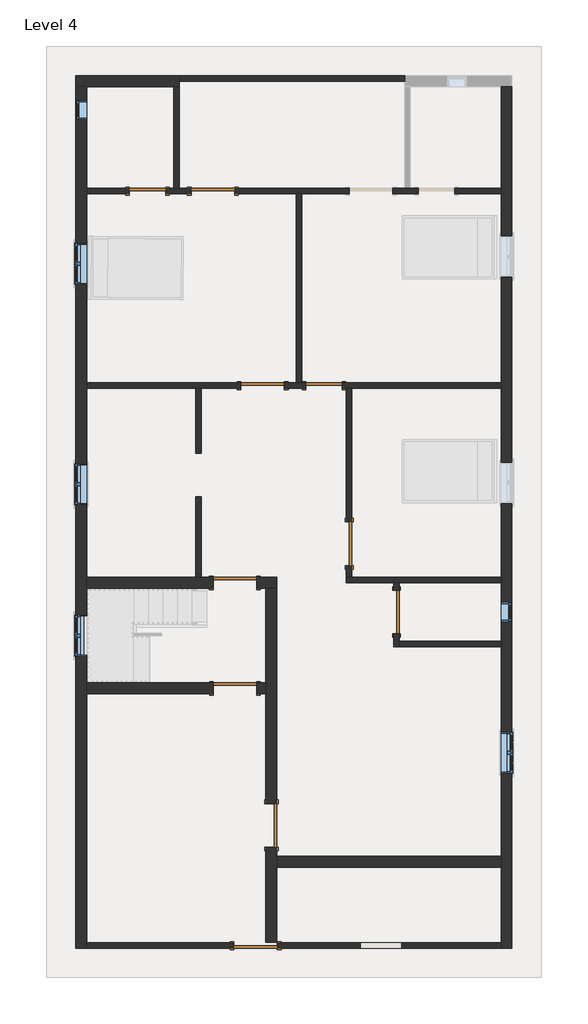
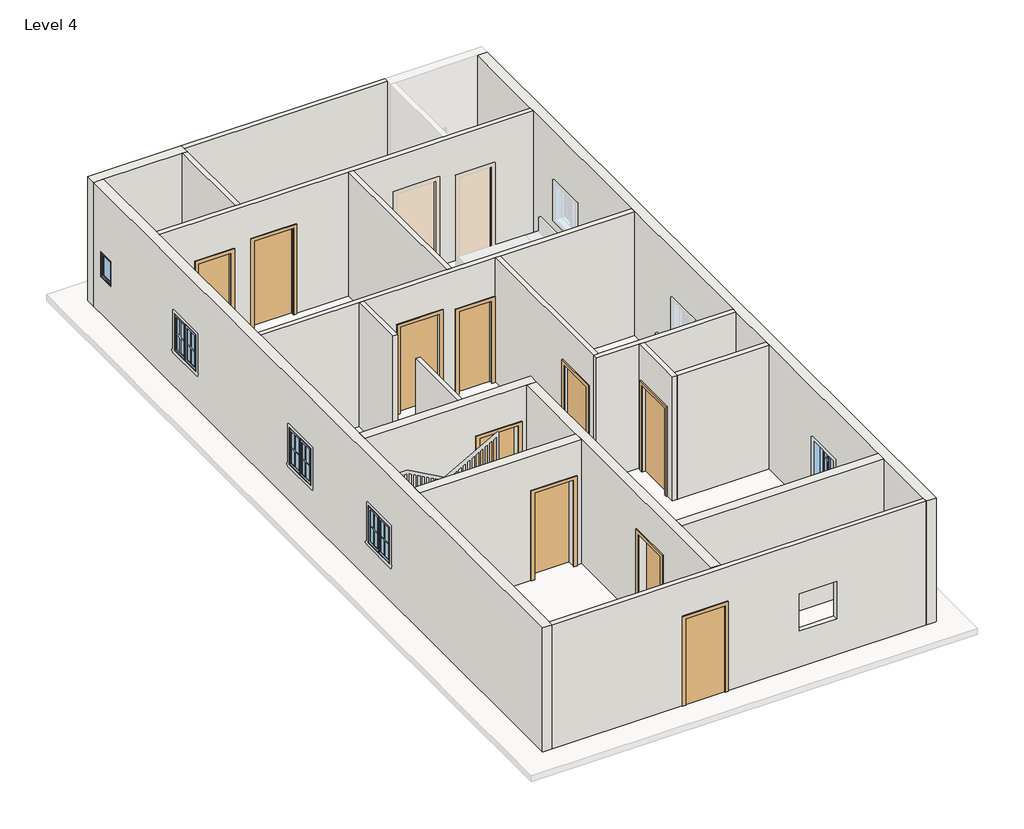
# One storey, part 1 of 3: 19 walls, 10 doors, 6 windows.
"""IFC4 building model written with IfcOpenShell, lengths in millimetres."""

from ifc_helpers import new_model, si_unit, frame, origin, place, context, project, spatial, polyline, outline, extrude, faceted_brep, transform, mapped, element, save
from components import door_d8f5dbb5, door_f2b275c1, door_e5f9f3c4, door_0ca8825f, door_305aa2a5, window_aa618e30, window_339605e1

model = new_model("IFC4")

# Units and contexts
model_context = context("Model", 3, world=origin())
ifc_project = project(units=[si_unit("LENGTHUNIT", "METRE", prefix="MILLI")], contexts=[model_context])

# Site, building, storey
site = spatial("IfcSite", under=ifc_project)
building = spatial("IfcBuilding", under=site)
storey = spatial("IfcBuildingStorey", under=building, Name="Level 4", Elevation=6400.8)

# Doors
placement = place(None, origin())
door_shape = door_d8f5dbb5(model_context)
element("IfcDoor", 1, ObjectType="Single-Flush : 30\" x 80\"", at=placement, inside=storey, context=model_context, shape_type="MappedRepresentation", body=[
    mapped(door_shape, transform((-4322.2915084, 8007.7072267, 6400.8), x_axis=(1.0, 0.0, 0.0), y_axis=(0.0, 1.0, 0.0), z_axis=(0.0, 0.0, 1.0))),
])
door_2_shape = door_f2b275c1(model_context)
element("IfcDoor", 2, ObjectType="Single-Flush : 30\" x 80\"", at=placement, inside=storey, context=model_context, shape_type="MappedRepresentation", body=[
    mapped(door_2_shape, transform((-621.124692, 3931.0072267, 6400.8), x_axis=(-1.0, 0.0, 0.0), y_axis=(0.0, -1.0, 0.0), z_axis=(0.0, 0.0, 1.0))),
])
door_3_shape = door_e5f9f3c4(model_context)
element("IfcDoor", 3, ObjectType="Single-Flush : 36\" x 84\"", at=placement, inside=storey, context=model_context, shape_type="MappedRepresentation", body=[
    mapped(door_3_shape, transform((-1909.2915084, 3931.0072267, 6400.8), x_axis=(1.0, 0.0, 0.0), y_axis=(0.0, 1.0, 0.0), z_axis=(0.0, 0.0, 1.0))),
])
element("IfcDoor", 4, ObjectType="Single-Flush : 36\" x 84\"", at=placement, inside=storey, context=model_context, shape_type="MappedRepresentation", body=[
    mapped(door_3_shape, transform((-94.9578757, 616.3072267, 6400.8), x_axis=(0.0, -1.0, 0.0), y_axis=(1.0, 0.0, 0.0), z_axis=(0.0, 0.0, 1.0))),
])
element("IfcDoor", 5, ObjectType="Single-Flush : 36\" x 84\"", at=placement, inside=storey, context=model_context, shape_type="MappedRepresentation", body=[
    mapped(door_3_shape, transform((-2055.3415084, -7803.7927733, 6400.8), x_axis=(-1.0, 0.0, 0.0), y_axis=(0.0, -1.0, 0.0), z_axis=(0.0, 0.0, 1.0))),
])
door_4_shape = door_0ca8825f(model_context)
element("IfcDoor", 6, ObjectType="Single-Flush : 36\" x 84\"", at=placement, inside=storey, context=model_context, shape_type="MappedRepresentation", body=[
    mapped(door_4_shape, transform((-2490.3165084, -202.8427733, 6400.8), x_axis=(1.0, 0.0, 0.0), y_axis=(0.0, 1.0, 0.0), z_axis=(0.0, 0.0, 1.0))),
])
element("IfcDoor", 7, ObjectType="Single-Flush : 36\" x 84\"", at=placement, inside=storey, context=model_context, shape_type="MappedRepresentation", body=[
    mapped(door_4_shape, transform((-2487.1415084, -2412.6427733, 6400.8), x_axis=(1.0, 0.0, 0.0), y_axis=(0.0, 1.0, 0.0), z_axis=(0.0, 0.0, 1.0))),
])
element("IfcDoor", 8, ObjectType="Single-Flush : 36\" x 84\"", at=placement, inside=storey, context=model_context, shape_type="MappedRepresentation", body=[
    mapped(door_4_shape, transform((-1725.1415084, -5282.8427733, 6400.8), x_axis=(0.0, -1.0, 0.0), y_axis=(1.0, 0.0, 0.0), z_axis=(0.0, 0.0, 1.0))),
])
door_5_shape = door_305aa2a5(model_context)
element("IfcDoor", 9, ObjectType="Single-Flush : 36\" x 84\"", at=placement, inside=storey, context=model_context, shape_type="MappedRepresentation", body=[
    mapped(door_5_shape, transform((897.4084916, -812.4427733, 6400.8), x_axis=(0.0, 1.0, 0.0), y_axis=(-1.0, 0.0, 0.0), z_axis=(0.0, 0.0, 1.0))),
])
element("IfcDoor", 10, ObjectType="Single-Flush : 36\" x 84\"", at=placement, inside=storey, context=model_context, shape_type="MappedRepresentation", body=[
    mapped(door_5_shape, transform((-2950.6915084, 8007.7072267, 6400.8), x_axis=(-1.0, 0.0, 0.0), y_axis=(0.0, -1.0, 0.0), z_axis=(0.0, 0.0, 1.0))),
])

# Walls
element("IfcWall", 11, ObjectType="WALL4.5\"", at=placement, inside=storey, context=model_context, shape_type="Brep", body=[
    faceted_brep([(821.2084916, 7950.5572267, 8534.4), (821.2084916, 7950.5572267, 6400.8), (1354.6084916, 7950.5572267, 6400.8), (1354.6084916, 7950.5572267, 8432.8), (2116.6084916, 7950.5572267, 8432.8), (2116.6084916, 7950.5572267, 6400.8), (3088.1584916, 7950.5572267, 6400.8), (3088.1584916, 7950.5572267, 9448.8), (-1090.1415084, 7950.5572267, 9448.8), (-1204.4415084, 7950.5572267, 9448.8), (-5598.6415084, 7950.5572267, 9448.8), (-5598.6415084, 7950.5572267, 6400.8), (-4703.2915084, 7950.5572267, 6400.8), (-4703.2915084, 7950.5572267, 8432.8), (-3941.2915084, 7950.5572267, 8432.8), (-3941.2915084, 7950.5572267, 6400.8), (-3407.8915084, 7950.5572267, 6400.8), (-3407.8915084, 7950.5572267, 8534.4), (-2493.4915084, 7950.5572267, 8534.4), (-2493.4915084, 7950.5572267, 6400.8), (-1204.4415084, 7950.5572267, 6400.8), (-1090.1415084, 7950.5572267, 6400.8), (-93.1915084, 7950.5572267, 6400.8), (-93.1915084, 7950.5572267, 8534.4), (1354.6084916, 8064.8572267, 6400.8), (1183.1584916, 8064.8572267, 6400.8), (1068.8584916, 8064.8572267, 6400.8), (821.2084916, 8064.8572267, 6400.8), (821.2084916, 8064.8572267, 8534.4), (-93.1915084, 8064.8572267, 8534.4), (-93.1915084, 8064.8572267, 6400.8), (-2493.4915084, 8064.8572267, 6400.8), (-2493.4915084, 8064.8572267, 8534.4), (-3407.8915084, 8064.8572267, 8534.4), (-3407.8915084, 8064.8572267, 6400.8), (-3655.5415084, 8064.8572267, 6400.8), (-3769.8415084, 8064.8572267, 6400.8), (-3941.2915084, 8064.8572267, 6400.8), (-3941.2915084, 8064.8572267, 8432.8), (-4703.2915084, 8064.8572267, 8432.8), (-4703.2915084, 8064.8572267, 6400.8), (-5598.6415084, 8064.8572267, 6400.8), (-5598.6415084, 8064.8572267, 9448.8), (-3769.8415084, 8064.8572267, 9448.8), (-3655.5415084, 8064.8572267, 9448.8), (1068.8584916, 8064.8572267, 9448.8), (1183.1584916, 8064.8572267, 9448.8), (3088.1584916, 8064.8572267, 9448.8), (3088.1584916, 8064.8572267, 6400.8), (2116.6084916, 8064.8572267, 6400.8), (2116.6084916, 8064.8572267, 8432.8), (1354.6084916, 8064.8572267, 8432.8)], [[[0, 1, 2, 3, 4, 5, 6, 7, 8, 9, 10, 11, 12, 13, 14, 15, 16, 17, 18, 19, 20, 21, 22, 23]], [[24, 25, 26, 27, 28, 29, 30, 31, 32, 33, 34, 35, 36, 37, 38, 39, 40, 41, 42, 43, 44, 45, 46, 47, 48, 49, 50, 51]], [[12, 11, 41, 40]], [[49, 48, 6, 5]], [[37, 36, 35, 34, 16, 15]], [[2, 1, 27, 26, 25, 24]], [[22, 21, 20, 19, 31, 30]], [[11, 10, 42, 41]], [[7, 6, 48, 47]], [[38, 37, 15, 14]], [[39, 38, 14, 13]], [[40, 39, 13, 12]], [[3, 2, 24, 51]], [[4, 3, 51, 50]], [[5, 4, 50, 49]], [[17, 16, 34, 33]], [[18, 17, 33, 32]], [[19, 18, 32, 31]], [[28, 27, 1, 0]], [[29, 28, 0, 23]], [[30, 29, 23, 22]], [[10, 9, 8, 7, 47, 46, 45, 44, 43, 42]]]),
])
element("IfcWall", 12, ObjectType="WALL4.5\"", at=placement, inside=storey, context=model_context, shape_type="SweptSolid", body=[
    extrude(outline(polyline([(-3769.8415084, 8064.8572267), (-3769.8415084, 10198.4572267), (-3655.5415084, 10198.4572267), (-3655.5415084, 8064.8572267), (-3769.8415084, 8064.8572267)])), frame((0.0, 0.0, 6400.8), z_axis=(0.0, 0.0, 1.0), x_axis=(1.0, 0.0, 0.0)), (0.0, 0.0, 1.0), 3048.0),
])
element("IfcWall", 13, ObjectType="WALL4.5\"", at=placement, inside=storey, context=model_context, shape_type="SweptSolid", body=[
    extrude(outline(polyline([(-1204.4415084, 3988.1572267), (-1204.4415084, 7950.5572267), (-1090.1415084, 7950.5572267), (-1090.1415084, 3988.1572267), (-1204.4415084, 3988.1572267)])), frame((0.0, 0.0, 6400.8), z_axis=(0.0, 0.0, 1.0), x_axis=(1.0, 0.0, 0.0)), (0.0, 0.0, 1.0), 3048.0),
])
element("IfcWall", 14, ObjectType="WALL4.5\"", at=placement, inside=storey, context=model_context, shape_type="Brep", body=[
    faceted_brep([(-1452.0915084, 3873.8572267, 6400.8), (-1002.124692, 3873.8572267, 6400.8), (-1002.124692, 3873.8572267, 8432.8), (-240.124692, 3873.8572267, 8432.8), (-240.124692, 3873.8572267, 6400.8), (-152.1078757, 3873.8572267, 6400.8), (-37.8078757, 3873.8572267, 6400.8), (3088.1584916, 3873.8572267, 6400.8), (3088.1584916, 3873.8572267, 9448.8), (-37.8078757, 3873.8572267, 9448.8), (-152.1078757, 3873.8572267, 9448.8), (-3198.3415084, 3873.8572267, 9448.8), (-3312.6415084, 3873.8572267, 9448.8), (-5598.6415084, 3873.8572267, 9448.8), (-5598.6415084, 3873.8572267, 6400.8), (-3312.6415084, 3873.8572267, 6400.8), (-3198.3415084, 3873.8572267, 6400.8), (-2366.4915084, 3873.8572267, 6400.8), (-2366.4915084, 3873.8572267, 8534.4), (-1452.0915084, 3873.8572267, 8534.4), (-1002.124692, 3988.1572267, 8432.8), (-1002.124692, 3988.1572267, 6400.8), (-1090.1415084, 3988.1572267, 6400.8), (-1204.4415084, 3988.1572267, 6400.8), (-1452.0915084, 3988.1572267, 6400.8), (-1452.0915084, 3988.1572267, 8534.4), (-2366.4915084, 3988.1572267, 8534.4), (-2366.4915084, 3988.1572267, 6400.8), (-5598.6415084, 3988.1572267, 6400.8), (-5598.6415084, 3988.1572267, 9448.8), (-1204.4415084, 3988.1572267, 9448.8), (-1090.1415084, 3988.1572267, 9448.8), (3088.1584916, 3988.1572267, 9448.8), (3088.1584916, 3988.1572267, 6400.8), (-240.124692, 3988.1572267, 6400.8), (-240.124692, 3988.1572267, 8432.8)], [[[0, 1, 2, 3, 4, 5, 6, 7, 8, 9, 10, 11, 12, 13, 14, 15, 16, 17, 18, 19]], [[20, 21, 22, 23, 24, 25, 26, 27, 28, 29, 30, 31, 32, 33, 34, 35]], [[17, 16, 15, 14, 28, 27]], [[34, 33, 7, 6, 5, 4]], [[24, 23, 22, 21, 1, 0]], [[14, 13, 29, 28]], [[8, 7, 33, 32]], [[25, 24, 0, 19]], [[26, 25, 19, 18]], [[27, 26, 18, 17]], [[2, 1, 21, 20]], [[3, 2, 20, 35]], [[4, 3, 35, 34]], [[13, 12, 11, 10, 9, 8, 32, 31, 30, 29]]]),
])
element("IfcWall", 15, ObjectType="WALL4.5\"", at=placement, inside=storey, context=model_context, shape_type="SweptSolid", body=[
    extrude(outline(polyline([(-3312.6415084, 2514.5843832), (-3312.6415084, 3873.8572267), (-3198.3415084, 3873.8572267), (-3198.3415084, 2514.5843832), (-3312.6415084, 2514.5843832)])), frame((0.0, 0.0, 6400.8), z_axis=(0.0, 0.0, 1.0), x_axis=(1.0, 0.0, 0.0)), (0.0, 0.0, 1.0), 3048.0),
])
element("IfcWall", 16, ObjectType="WALL4.5\"", at=placement, inside=storey, context=model_context, shape_type="SweptSolid", body=[
    extrude(outline(polyline([(-3312.6415084, -88.5427733), (-3312.6415084, 1600.2092553), (-3198.3415084, 1600.2092553), (-3198.3415084, -88.5427733), (-3312.6415084, -88.5427733)])), frame((0.0, 0.0, 6400.8), z_axis=(0.0, 0.0, 1.0), x_axis=(1.0, 0.0, 0.0)), (0.0, 0.0, 1.0), 3048.0),
])
element("IfcWall", 17, ObjectType="WALL4.5\"", at=placement, inside=storey, context=model_context, shape_type="SweptSolid", body=[
    extrude(outline(polyline([(159.1072267, 8534.4), (159.1072267, 6400.8), (-88.5427733, 6400.8), (-88.5427733, 9448.8), (3873.8572267, 9448.8), (3873.8572267, 6400.8), (1073.5072267, 6400.8), (1073.5072267, 8534.4), (159.1072267, 8534.4)])), frame((-152.1078757, 0.0, 0.0), z_axis=(1.0, 0.0, 0.0), x_axis=(0.0, 1.0, 0.0)), (0.0, 0.0, 1.0), 114.3),
])
element("IfcWall", 18, ObjectType="WALL4.5\"", at=placement, inside=storey, context=model_context, shape_type="Brep", body=[
    faceted_brep([(-152.1078757, -202.8427733, 6400.8), (840.2584916, -202.8427733, 6400.8), (954.5584916, -202.8427733, 6400.8), (3088.1584916, -202.8427733, 6400.8), (3088.1584916, -202.8427733, 9448.8), (954.5584916, -202.8427733, 9448.8), (840.2584916, -202.8427733, 9448.8), (-152.1078757, -202.8427733, 9448.8), (-152.1078757, -88.5427733, 6400.8), (-152.1078757, -88.5427733, 9448.8), (-37.8078757, -88.5427733, 9448.8), (3088.1584916, -88.5427733, 9448.8), (3088.1584916, -88.5427733, 6400.8), (-37.8078757, -88.5427733, 6400.8)], [[[0, 1, 2, 3, 4, 5, 6, 7]], [[8, 9, 10, 11, 12, 13]], [[3, 2, 1, 0, 8, 13, 12]], [[4, 3, 12, 11]], [[0, 7, 9, 8]], [[7, 6, 5, 4, 11, 10, 9]]]),
])
element("IfcWall", 19, ObjectType="WALL4.5\"", at=placement, inside=storey, context=model_context, shape_type="Brep", body=[
    faceted_brep([(840.2584916, -202.8427733, 6400.8), (840.2584916, -355.2427733, 6400.8), (840.2584916, -355.2427733, 8534.4), (840.2584916, -1269.6427733, 8534.4), (840.2584916, -1269.6427733, 6400.8), (840.2584916, -1536.3427733, 6400.8), (840.2584916, -1536.3427733, 9448.8), (840.2584916, -202.8427733, 9448.8), (954.5584916, -355.2427733, 8534.4), (954.5584916, -355.2427733, 6400.8), (954.5584916, -202.8427733, 6400.8), (954.5584916, -202.8427733, 9448.8), (954.5584916, -1422.0427733, 9448.8), (954.5584916, -1536.3427733, 9448.8), (954.5584916, -1536.3427733, 6400.8), (954.5584916, -1422.0427733, 6400.8), (954.5584916, -1269.6427733, 6400.8), (954.5584916, -1269.6427733, 8534.4)], [[[0, 1, 2, 3, 4, 5, 6, 7]], [[8, 9, 10, 11, 12, 13, 14, 15, 16, 17]], [[10, 9, 1, 0]], [[16, 15, 14, 5, 4]], [[0, 7, 11, 10]], [[6, 5, 14, 13]], [[2, 1, 9, 8]], [[3, 2, 8, 17]], [[4, 3, 17, 16]], [[7, 6, 13, 12, 11]]]),
])
element("IfcWall", 20, ObjectType="WALL4.5\"", at=placement, inside=storey, context=model_context, shape_type="SweptSolid", body=[
    extrude(outline(polyline([(3088.1584916, -1536.3427733), (954.5584916, -1536.3427733), (954.5584916, -1422.0427733), (3088.1584916, -1422.0427733), (3088.1584916, -1536.3427733)])), frame((0.0, 0.0, 6400.8), z_axis=(0.0, 0.0, 1.0), x_axis=(1.0, 0.0, 0.0)), (0.0, 0.0, 1.0), 3048.0),
])
element("IfcWall", 21, ObjectType="WALL4.5\"", at=placement, inside=storey, context=model_context, shape_type="SweptSolid", body=[
    extrude(outline(polyline([(6400.8, -5598.6415084), (6400.8, -2512.5415084), (8534.4, -2512.5415084), (8534.4, -1598.1415084), (6400.8, -1598.1415084), (6400.8, 3088.1584916), (9448.8, 3088.1584916), (9448.8, -5598.6415084), (6400.8, -5598.6415084)]), holes=[polyline([(8199.7190366, 141.7584916), (8199.7190366, 1005.3584916), (7285.3190366, 1005.3584916), (7285.3190366, 141.7584916), (8199.7190366, 141.7584916)])]), frame((0.0, -7860.9427733, 0.0), z_axis=(0.0, 1.0, 0.0), x_axis=(0.0, 0.0, 1.0)), (0.0, 0.0, 1.0), 114.3),
])
element("IfcWall", 22, ObjectType="WALL4.5\"", at=placement, inside=storey, context=model_context, shape_type="SweptSolid", body=[
    extrude(outline(polyline([(1068.8584916, 10312.7572267), (-3655.5415084, 10312.7572267), (-3655.5415084, 10427.0572267), (1068.8584916, 10427.0572267), (1068.8584916, 10312.7572267)])), frame((0.0, 0.0, 6400.8), z_axis=(0.0, 0.0, 1.0), x_axis=(1.0, 0.0, 0.0)), (0.0, 0.0, 1.0), 3048.0),
])
element("IfcWall", 23, ObjectType="WALL9\"", at=placement, inside=storey, context=model_context, shape_type="Brep", body=[
    faceted_brep([(-3655.5415084, 10427.0572267, 6400.8), (-5827.2415084, 10427.0572267, 6400.8), (-5827.2415084, 10427.0572267, 9448.8), (-3655.5415084, 10427.0572267, 9448.8), (-3655.5415084, 10198.4572267, 6400.8), (-3655.5415084, 10198.4572267, 9448.8), (-3769.8415084, 10198.4572267, 9448.8), (-5598.6415084, 10198.4572267, 9448.8), (-5827.2415084, 10198.4572267, 9448.8), (-5827.2415084, 10198.4572267, 6400.8), (-5598.6415084, 10198.4572267, 6400.8), (-3769.8415084, 10198.4572267, 6400.8), (-3655.5415084, 10312.7572267, 6400.8), (-3655.5415084, 10312.7572267, 9448.8)], [[[0, 1, 2, 3]], [[4, 5, 6, 7, 8, 9, 10, 11]], [[1, 0, 12, 4, 11, 10, 9]], [[2, 1, 9, 8]], [[0, 3, 13, 5, 4, 12]], [[3, 2, 8, 7, 6, 5, 13]]]),
])
element("IfcWall", 24, ObjectType="WALL9\"", at=placement, inside=storey, context=model_context, shape_type="Brep", body=[
    faceted_brep([(-5827.2415084, 10198.4572267, 6400.8), (-5827.2415084, -7860.9427733, 6400.8), (-5827.2415084, -7860.9427733, 9448.8), (-5827.2415084, 10198.4572267, 9448.8), (-5827.2415084, 9906.3572267, 7924.8), (-5827.2415084, 9499.9572267, 7924.8), (-5827.2415084, 9499.9572267, 7315.2), (-5827.2415084, 9906.3572267, 7315.2), (-5827.2415084, 6915.5072267, 8229.6), (-5827.2415084, 6051.9072267, 8229.6), (-5827.2415084, 6051.9072267, 7315.2), (-5827.2415084, 6915.5072267, 7315.2), (-5827.2415084, 2295.8822267, 8229.6), (-5827.2415084, 1432.2822267, 8229.6), (-5827.2415084, 1432.2822267, 7315.2), (-5827.2415084, 2295.8822267, 7315.2), (-5827.2415084, -875.9427733, 8229.6), (-5827.2415084, -1739.5427733, 8229.6), (-5827.2415084, -1739.5427733, 7315.2), (-5827.2415084, -875.9427733, 7315.2), (-5598.6415084, 10198.4572267, 6400.8), (-5598.6415084, 10198.4572267, 9448.8), (-5598.6415084, 8064.8572267, 9448.8), (-5598.6415084, 7950.5572267, 9448.8), (-5598.6415084, 3988.1572267, 9448.8), (-5598.6415084, 3873.8572267, 9448.8), (-5598.6415084, -88.5427733, 9448.8), (-5598.6415084, -317.1427733, 9448.8), (-5598.6415084, -2298.3427733, 9448.8), (-5598.6415084, -2526.9427733, 9448.8), (-5598.6415084, -7746.6427733, 9448.8), (-5598.6415084, -7860.9427733, 9448.8), (-5598.6415084, -7860.9427733, 6400.8), (-5598.6415084, -7746.6427733, 6400.8), (-5598.6415084, -2526.9427733, 6400.8), (-5598.6415084, -2298.3427733, 6400.8), (-5598.6415084, -317.1427733, 6400.8), (-5598.6415084, -88.5427733, 6400.8), (-5598.6415084, 3873.8572267, 6400.8), (-5598.6415084, 3988.1572267, 6400.8), (-5598.6415084, 7950.5572267, 6400.8), (-5598.6415084, 8064.8572267, 6400.8), (-5598.6415084, 9906.3572267, 7924.8), (-5598.6415084, 9906.3572267, 7315.2), (-5598.6415084, 9499.9572267, 7315.2), (-5598.6415084, 9499.9572267, 7924.8), (-5598.6415084, 6915.5072267, 8229.6), (-5598.6415084, 6915.5072267, 7315.2), (-5598.6415084, 6051.9072267, 7315.2), (-5598.6415084, 6051.9072267, 8229.6), (-5598.6415084, 2295.8822267, 8229.6), (-5598.6415084, 2295.8822267, 7315.2), (-5598.6415084, 1432.2822267, 7315.2), (-5598.6415084, 1432.2822267, 8229.6), (-5598.6415084, -875.9427733, 8229.6), (-5598.6415084, -875.9427733, 7315.2), (-5598.6415084, -1739.5427733, 7315.2), (-5598.6415084, -1739.5427733, 8229.6)], [[[0, 1, 2, 3], [4, 5, 6, 7], [8, 9, 10, 11], [12, 13, 14, 15], [16, 17, 18, 19]], [[20, 21, 22, 23, 24, 25, 26, 27, 28, 29, 30, 31, 32, 33, 34, 35, 36, 37, 38, 39, 40, 41], [42, 43, 44, 45], [46, 47, 48, 49], [50, 51, 52, 53], [54, 55, 56, 57]], [[1, 0, 20, 41, 40, 39, 38, 37, 36, 35, 34, 33, 32]], [[0, 3, 21, 20]], [[2, 1, 32, 31]], [[43, 42, 4, 7]], [[44, 43, 7, 6]], [[45, 44, 6, 5]], [[42, 45, 5, 4]], [[47, 46, 8, 11]], [[48, 47, 11, 10]], [[49, 48, 10, 9]], [[46, 49, 9, 8]], [[51, 50, 12, 15]], [[52, 51, 15, 14]], [[53, 52, 14, 13]], [[50, 53, 13, 12]], [[55, 54, 16, 19]], [[56, 55, 19, 18]], [[57, 56, 18, 17]], [[54, 57, 17, 16]], [[3, 2, 31, 30, 29, 28, 27, 26, 25, 24, 23, 22, 21]]]),
])
element("IfcWall", 25, ObjectType="WALL9\"", at=placement, inside=storey, context=model_context, shape_type="Brep", body=[
    faceted_brep([(3088.1584916, 10198.4572267, 6400.8), (3088.1584916, 8064.8572267, 6400.8), (3088.1584916, 7950.5572267, 6400.8), (3088.1584916, 3988.1572267, 6400.8), (3088.1584916, 3873.8572267, 6400.8), (3088.1584916, -88.5427733, 6400.8), (3088.1584916, -202.8427733, 6400.8), (3088.1584916, -1422.0427733, 6400.8), (3088.1584916, -1536.3427733, 6400.8), (3088.1584916, -5930.5427733, 6400.8), (3088.1584916, -6159.1427733, 6400.8), (3088.1584916, -7746.6427733, 6400.8), (3088.1584916, -7860.9427733, 6400.8), (3088.1584916, -7860.9427733, 9448.8), (3088.1584916, -7746.6427733, 9448.8), (3088.1584916, -6159.1427733, 9448.8), (3088.1584916, -5930.5427733, 9448.8), (3088.1584916, -1536.3427733, 9448.8), (3088.1584916, -1422.0427733, 9448.8), (3088.1584916, -202.8427733, 9448.8), (3088.1584916, -88.5427733, 9448.8), (3088.1584916, 3873.8572267, 9448.8), (3088.1584916, 3988.1572267, 9448.8), (3088.1584916, 7950.5572267, 9448.8), (3088.1584916, 8064.8572267, 9448.8), (3088.1584916, 10198.4572267, 9448.8), (3088.1584916, -1015.6427733, 7924.8), (3088.1584916, -1015.6427733, 7315.2), (3088.1584916, -609.2427733, 7315.2), (3088.1584916, -609.2427733, 7924.8), (3088.1584916, 6204.3072267, 8229.6), (3088.1584916, 6204.3072267, 7315.2), (3088.1584916, 7067.9072267, 7315.2), (3088.1584916, 7067.9072267, 8229.6), (3088.1584916, 1460.8572267, 8229.6), (3088.1584916, 1460.8572267, 7315.2), (3088.1584916, 2324.4572267, 7315.2), (3088.1584916, 2324.4572267, 8229.6), (3088.1584916, -4193.8177733, 8229.6), (3088.1584916, -4193.8177733, 7315.2), (3088.1584916, -3330.2177733, 7315.2), (3088.1584916, -3330.2177733, 8229.6), (3316.7584916, 10198.4572267, 6400.8), (3316.7584916, 10198.4572267, 9448.8), (3316.7584916, -7860.9427733, 9448.8), (3316.7584916, -7860.9427733, 6400.8), (3316.7584916, -1015.6427733, 7924.8), (3316.7584916, -609.2427733, 7924.8), (3316.7584916, -609.2427733, 7315.2), (3316.7584916, -1015.6427733, 7315.2), (3316.7584916, 6204.3072267, 8229.6), (3316.7584916, 7067.9072267, 8229.6), (3316.7584916, 7067.9072267, 7315.2), (3316.7584916, 6204.3072267, 7315.2), (3316.7584916, 1460.8572267, 8229.6), (3316.7584916, 2324.4572267, 8229.6), (3316.7584916, 2324.4572267, 7315.2), (3316.7584916, 1460.8572267, 7315.2), (3316.7584916, -4193.8177733, 8229.6), (3316.7584916, -3330.2177733, 8229.6), (3316.7584916, -3330.2177733, 7315.2), (3316.7584916, -4193.8177733, 7315.2)], [[[0, 1, 2, 3, 4, 5, 6, 7, 8, 9, 10, 11, 12, 13, 14, 15, 16, 17, 18, 19, 20, 21, 22, 23, 24, 25], [26, 27, 28, 29], [30, 31, 32, 33], [34, 35, 36, 37], [38, 39, 40, 41]], [[42, 43, 44, 45], [46, 47, 48, 49], [50, 51, 52, 53], [54, 55, 56, 57], [58, 59, 60, 61]], [[12, 11, 10, 9, 8, 7, 6, 5, 4, 3, 2, 1, 0, 42, 45]], [[0, 25, 43, 42]], [[13, 12, 45, 44]], [[27, 26, 46, 49]], [[28, 27, 49, 48]], [[29, 28, 48, 47]], [[26, 29, 47, 46]], [[31, 30, 50, 53]], [[32, 31, 53, 52]], [[33, 32, 52, 51]], [[30, 33, 51, 50]], [[35, 34, 54, 57]], [[36, 35, 57, 56]], [[37, 36, 56, 55]], [[34, 37, 55, 54]], [[39, 38, 58, 61]], [[40, 39, 61, 60]], [[41, 40, 60, 59]], [[38, 41, 59, 58]], [[25, 24, 23, 22, 21, 20, 19, 18, 17, 16, 15, 14, 13, 44, 43]]]),
])
element("IfcWall", 26, ObjectType="WALL9\"", at=placement, inside=storey, context=model_context, shape_type="Brep", body=[
    faceted_brep([(-2033.1165084, -317.1427733, 8534.4), (-2033.1165084, -317.1427733, 6400.8), (-1839.4415084, -317.1427733, 6400.8), (-1610.8415084, -317.1427733, 6400.8), (-1610.8415084, -317.1427733, 9448.8), (-1839.4415084, -317.1427733, 9448.8), (-5598.6415084, -317.1427733, 9448.8), (-5598.6415084, -317.1427733, 6400.8), (-2947.5165084, -317.1427733, 6400.8), (-2947.5165084, -317.1427733, 8534.4), (-1610.8415084, -88.5427733, 6400.8), (-2033.1165084, -88.5427733, 6400.8), (-2033.1165084, -88.5427733, 8534.4), (-2947.5165084, -88.5427733, 8534.4), (-2947.5165084, -88.5427733, 6400.8), (-3198.3415084, -88.5427733, 6400.8), (-3312.6415084, -88.5427733, 6400.8), (-5598.6415084, -88.5427733, 6400.8), (-5598.6415084, -88.5427733, 9448.8), (-3312.6415084, -88.5427733, 9448.8), (-3198.3415084, -88.5427733, 9448.8), (-1610.8415084, -88.5427733, 9448.8)], [[[0, 1, 2, 3, 4, 5, 6, 7, 8, 9]], [[10, 11, 12, 13, 14, 15, 16, 17, 18, 19, 20, 21]], [[8, 7, 17, 16, 15, 14]], [[3, 2, 1, 11, 10]], [[7, 6, 18, 17]], [[4, 3, 10, 21]], [[12, 11, 1, 0]], [[13, 12, 0, 9]], [[14, 13, 9, 8]], [[6, 5, 4, 21, 20, 19, 18]]]),
])
element("IfcWall", 27, ObjectType="WALL9\"", at=placement, inside=storey, context=model_context, shape_type="Brep", body=[
    faceted_brep([(-1839.4415084, -5740.0427733, 8534.4), (-1839.4415084, -5740.0427733, 6400.8), (-1839.4415084, -7733.9427733, 6400.8), (-1839.4415084, -7733.9427733, 9448.8), (-1839.4415084, -2526.9427733, 9448.8), (-1839.4415084, -2298.3427733, 9448.8), (-1839.4415084, -317.1427733, 9448.8), (-1839.4415084, -317.1427733, 6400.8), (-1839.4415084, -2298.3427733, 6400.8), (-1839.4415084, -2526.9427733, 6400.8), (-1839.4415084, -4825.6427733, 6400.8), (-1839.4415084, -4825.6427733, 8534.4), (-1610.8415084, -7733.9427733, 6400.8), (-1610.8415084, -6159.1427733, 6400.8), (-1610.8415084, -5930.5427733, 6400.8), (-1610.8415084, -5740.0427733, 6400.8), (-1610.8415084, -5740.0427733, 8534.4), (-1610.8415084, -4825.6427733, 8534.4), (-1610.8415084, -4825.6427733, 6400.8), (-1610.8415084, -317.1427733, 6400.8), (-1610.8415084, -317.1427733, 9448.8), (-1610.8415084, -5930.5427733, 9448.8), (-1610.8415084, -6159.1427733, 9448.8), (-1610.8415084, -7733.9427733, 9448.8)], [[[0, 1, 2, 3, 4, 5, 6, 7, 8, 9, 10, 11]], [[12, 13, 14, 15, 16, 17, 18, 19, 20, 21, 22, 23]], [[2, 1, 15, 14, 13, 12]], [[10, 9, 8, 7, 19, 18]], [[3, 2, 12, 23]], [[7, 6, 20, 19]], [[16, 15, 1, 0]], [[17, 16, 0, 11]], [[18, 17, 11, 10]], [[6, 5, 4, 3, 23, 22, 21, 20]]]),
])
element("IfcWall", 28, ObjectType="WALL9\"", at=placement, inside=storey, context=model_context, shape_type="SweptSolid", body=[
    extrude(outline(polyline([(3088.1584916, -6159.1427733), (-1610.8415084, -6159.1427733), (-1610.8415084, -5930.5427733), (3088.1584916, -5930.5427733), (3088.1584916, -6159.1427733)])), frame((0.0, 0.0, 6400.8), z_axis=(0.0, 0.0, 1.0), x_axis=(1.0, 0.0, 0.0)), (0.0, 0.0, 1.0), 3048.0),
])
element("IfcWall", 29, ObjectType="WALL9\"", at=placement, inside=storey, context=model_context, shape_type="SweptSolid", body=[
    extrude(outline(polyline([(8534.4, -2029.9415084), (6400.8, -2029.9415084), (6400.8, -1839.4415084), (9448.8, -1839.4415084), (9448.8, -5598.6415084), (6400.8, -5598.6415084), (6400.8, -2944.3415084), (8534.4, -2944.3415084), (8534.4, -2029.9415084)])), frame((0.0, -2526.9427733, 0.0), z_axis=(0.0, 1.0, 0.0), x_axis=(0.0, 0.0, 1.0)), (0.0, 0.0, 1.0), 228.6),
])

# Windows
window_shape = window_aa618e30(model_context)
element("IfcWindow", 30, ObjectType="Fixed : 16\" x 24\"", at=placement, inside=storey, context=model_context, shape_type="MappedRepresentation", body=[
    mapped(window_shape, transform((-5712.9415084, 9741.2572267, 6400.8), x_axis=(0.0, 1.0, 0.0), y_axis=(-1.0, 0.0, 0.0), z_axis=(0.0, 0.0, 1.0))),
])
element("IfcWindow", 31, ObjectType="Fixed : 16\" x 24\"", at=placement, inside=storey, context=model_context, shape_type="MappedRepresentation", body=[
    mapped(window_shape, transform((3202.4584916, -850.5427733, 6400.8), x_axis=(0.0, -1.0, 0.0), y_axis=(1.0, 0.0, 0.0), z_axis=(0.0, 0.0, 1.0))),
])
window_2_shape = window_339605e1(model_context)
element("IfcWindow", 32, ObjectType="Window-Casement-Double : 34\" x 36\"", at=placement, inside=storey, context=model_context, shape_type="MappedRepresentation", body=[
    mapped(window_2_shape, transform((-5712.9415084, 6483.7072267, 6400.8), x_axis=(0.0, 1.0, 0.0), y_axis=(-1.0, 0.0, 0.0), z_axis=(0.0, 0.0, 1.0))),
])
element("IfcWindow", 33, ObjectType="Window-Casement-Double : 34\" x 36\"", at=placement, inside=storey, context=model_context, shape_type="MappedRepresentation", body=[
    mapped(window_2_shape, transform((-5712.9415084, 1864.0822267, 6400.8), x_axis=(0.0, 1.0, 0.0), y_axis=(-1.0, 0.0, 0.0), z_axis=(0.0, 0.0, 1.0))),
])
element("IfcWindow", 34, ObjectType="Window-Casement-Double : 34\" x 36\"", at=placement, inside=storey, context=model_context, shape_type="MappedRepresentation", body=[
    mapped(window_2_shape, transform((3202.4584916, -3762.0177733, 6400.8), x_axis=(0.0, -1.0, 0.0), y_axis=(1.0, 0.0, 0.0), z_axis=(0.0, 0.0, 1.0))),
])
element("IfcWindow", 35, ObjectType="Window-Casement-Double : 34\" x 36\"", at=placement, inside=storey, context=model_context, shape_type="MappedRepresentation", body=[
    mapped(window_2_shape, transform((-5712.9415084, -1307.7427733, 6400.8), x_axis=(0.0, 1.0, 0.0), y_axis=(-1.0, 0.0, 0.0), z_axis=(0.0, 0.0, 1.0))),
])

save(model, "model.ifc")

# Revit data of these elements
# Type "Single-Flush : 30\" x 80\""
#   Type Mark = "5"
#   Construction Type Id = "MDOOR"
#   Assembly Code = "C1020"
#   Analytic Construction = "Metal"
#   Thickness = 0' - 2"
#   Heat Transfer Coefficient (U) = 0.651978 BTU/(h·ft²·°F)
#   Height = 6' - 8"
#   Trim Projection Ext = 0' - 1"
#   Trim Projection Int = 0' - 1"
#   Trim Width = 0' - 3"
#   Width = 2' - 6"
#   Define Thermal Properties by = 1
#   Define Thermal Properties by = 1
#   Door Material = Door - Panel
#   Frame Material = Door - Frame
#   Visual Light Transmittance = 0
#   Solar Heat Gain Coefficient = 0
#   Function = (empty or 0)
#   Wall Closure = (empty or 0)
# Type "Single-Flush : 36\" x 84\""
#   Type Mark = "1"
#   Construction Type Id = "MDOOR"
#   Assembly Code = "C1020"
#   Analytic Construction = "Metal"
#   Thickness = 0' - 2"
#   Heat Transfer Coefficient (U) = 0.651978 BTU/(h·ft²·°F)
#   Height = 7' - 0"
#   Trim Projection Ext = 0' - 1"
#   Trim Projection Int = 0' - 1"
#   Trim Width = 0' - 3"
#   Width = 3' - 0"
#   Define Thermal Properties by = 1
#   Define Thermal Properties by = 1
#   Door Material = Door - Panel
#   Frame Material = Door - Frame
#   Visual Light Transmittance = 0
#   Solar Heat Gain Coefficient = 0
#   Function = (empty or 0)
#   Wall Closure = (empty or 0)
# Type "WALL4.5\""
#   Assembly Code = "B2010"
#   Layers, outside or top first: 0' - 4 1/2" no material (function 1)
# Type "WALL9\""
#   Assembly Code = "B2010"
#   Layers, outside or top first: 0' - 9" no material (function 1)
# Type "Fixed : 16\" x 24\""
#   Type Mark = "4"
#   Construction Type Id = "GSP4R"
#   Assembly Code = "B2020100"
#   Analytic Construction = "1/8 in Pilkington single glazing"
#   Visual Light Transmittance = 0.9
#   Solar Heat Gain Coefficient = 0.78
#   Heat Transfer Coefficient (U) = 0.6496 BTU/(h·ft²·°F)
#   Height = 2' - 0"
#   Default Sill Height = 3' - 0"
#   Width = 1' - 4"
#   Window Inset = 0' - 0 3/4"
#   Define Thermal Properties by = 1
#   Define Thermal Properties by = 1
#   Glass Pane Material = Glass
#   Sash Material = Sash
#   Wall Closure = (empty or 0)
# Type "Window-Casement-Double : 34\" x 36\""
#   Type Mark = "14"
#   Fire Rating = "0.5h"
#   Assembly Code = "B2020100"
#   Analytic Construction = "Double glazing - domestic"
#   Frame Extension [instance default] = 0' - 0 1/4"
#   Window Inset [instance default] = 0' - 0"
#   Wall Thickness [instance default] = 0' - 6"
#   Interior Wall Closure [instance default] = 0' - 2 1/4"
#   Half Width = 1' - 5"
#   Visual Light Transmittance = 0.81
#   Thermal Resistance (R) = 1.8146 (h·ft²·°F)/BTU
#   Solar Heat Gain Coefficient = 0.76
#   Rough Width = 2' - 10 1/2"
#   Rough Height = 3' - 0 1/2"
#   Height = 3' - 0"
#   Heat Transfer Coefficient (U) = 0.5511 BTU/(h·ft²·°F)
#   Exterior Wall Closure [instance default] = 0' - 1 1/4"
#   Extension Jamb [instance default] = 0' - 2 1/4"
#   Default Sill Height = 3' - 0"
#   Width = 2' - 10"
#   Define Thermal Properties by = 0
#   Muntin Visibility = yes
#   Interior Trim Visibility [instance default] = yes
#   Exterior Trim Visibility [instance default] = yes
#   Extension Jamb Visibility [instance default] = yes
#   Interior Trim Material = Wood - Stained
#   Muntin Pattern = Muntin Pattern_2x2 : Muntin Pattern_2x2
#   Interior Trim = Trim-Window-Interior-Flat : Picture Frame
#   Interior Frame Material = Wood - Stained
#   Glass Panel Material = Glass
#   Exterior Trim Material = Clad - White
#   Exterior Trim = Trim-Window-Exterior-Flat : with Sill
#   Exterior Frame Material = Clad - White
#   Wall Closure = (empty or 0)
# Elements 1, 2 (IfcDoor, "Single-Flush : 30\" x 80\"")
#   Phase Created = New Construction
#   Materials on its faces: "Door - Frame", "Door - Panel"
# Elements 3, 4, 5, 6, 7, 8, 9, 10 (IfcDoor, "Single-Flush : 36\" x 84\"")
#   Phase Created = New Construction
#   Materials on its faces: "Door - Frame", "Door - Panel"
# Elements 11, 21, 22 (IfcWall, "WALL4.5\"")
#   Top Offset = 0' - 0"
#   Base Offset = 0' - 0"
#   Unconnected Height = 10' - 0"
#   wall height = 10' - 0"
#   Phase Created = New Construction
#   Base Constraint = Level 4
#   Materials on its faces: "Default Wall", "Wood Planks"
# Elements 12, 13, 14, 15, 16, 17, 18, 19, 20 (IfcWall, "WALL4.5\"")
#   Top Offset = 0' - 0"
#   Base Offset = 0' - 0"
#   Unconnected Height = 10' - 0"
#   wall height = 10' - 0"
#   Phase Created = New Construction
#   Base Constraint = Level 4
#   Materials on its faces: "Default Wall"
# Elements 23, 24, 25 (IfcWall, "WALL9\"")
#   Top Offset = 0' - 0"
#   Base Offset = 0' - 0"
#   Unconnected Height = 10' - 0"
#   wall height = 10' - 0"
#   Phase Created = New Construction
#   Base Constraint = Level 4
#   Materials on its faces: "Default Wall", "Wood Planks"
# Elements 26, 27, 28, 29 (IfcWall, "WALL9\"")
#   Top Offset = 0' - 0"
#   Base Offset = 0' - 0"
#   Unconnected Height = 10' - 0"
#   wall height = 10' - 0"
#   Phase Created = New Construction
#   Base Constraint = Level 4
#   Materials on its faces: "Default Wall"
# Element 30 (IfcWindow, "Fixed : 16\" x 24\"")
#   Mark = "19"
#   Phase Created = New Construction
#   Materials on its faces: "Sash", "Glass"
# Element 31 (IfcWindow, "Fixed : 16\" x 24\"")
#   Mark = "21"
#   Phase Created = New Construction
#   Materials on its faces: "Sash", "Glass"
# Element 32 (IfcWindow, "Window-Casement-Double : 34\" x 36\"")
#   Mark = "24"
#   Window Inset = 0' - 0"
#   Interior Wall Closure = 0' - 2 1/4"
#   Frame Extension = 0' - 0 1/4"
#   Exterior Wall Closure = 0' - 1 1/4"
#   Interior Trim Visibility = yes
#   Exterior Trim Visibility = yes
#   Phase Created = New Construction
#   Materials on its faces: "Wood - Stained", "Glass", "Clad - White"
# Element 33 (IfcWindow, "Window-Casement-Double : 34\" x 36\"")
#   Mark = "25"
#   Window Inset = 0' - 0"
#   Interior Wall Closure = 0' - 2 1/4"
#   Frame Extension = 0' - 0 1/4"
#   Exterior Wall Closure = 0' - 1 1/4"
#   Interior Trim Visibility = yes
#   Exterior Trim Visibility = yes
#   Phase Created = New Construction
#   Materials on its faces: "Wood - Stained", "Glass", "Clad - White"
# Element 34 (IfcWindow, "Window-Casement-Double : 34\" x 36\"")
#   Mark = "26"
#   Window Inset = 0' - 0"
#   Interior Wall Closure = 0' - 2 1/4"
#   Frame Extension = 0' - 0 1/4"
#   Exterior Wall Closure = 0' - 1 1/4"
#   Interior Trim Visibility = yes
#   Exterior Trim Visibility = yes
#   Phase Created = New Construction
#   Materials on its faces: "Wood - Stained", "Glass", "Clad - White"
# Element 35 (IfcWindow, "Window-Casement-Double : 34\" x 36\"")
#   Mark = "27"
#   Window Inset = 0' - 0"
#   Interior Wall Closure = 0' - 2 1/4"
#   Frame Extension = 0' - 0 1/4"
#   Exterior Wall Closure = 0' - 1 1/4"
#   Interior Trim Visibility = yes
#   Exterior Trim Visibility = yes
#   Phase Created = New Construction
#   Materials on its faces: "Wood - Stained", "Glass", "Clad - White"
# Materials
#   "Door - Panel": class "Wood", colour RGB 210 159 95, transparency 0, Cost = 0
#   "Door - Frame": colour RGB 118 70 51, transparency 0, Cost = 0
#   "Glass": class "Glass", colour RGB 0 128 192, transparency 0.75, Description = "Soda Lime Glass", Cost = 0
#   "Sash": class "Wood", colour RGB 224 178 126, transparency 0, Cost = 0
#   "Wood - Stained": class "Wood", colour RGB 224 178 126, transparency 0, Cost = 0
#   "Clad - White": class "Wood", colour RGB 242 242 238, transparency 0, Cost = 0
#   "Default Wall": colour RGB 128 128 128, transparency 0, Cost = 0
#   "Wood Planks": class "Wood", colour RGB 193 160 115, transparency 0, Description = "Physical material.", Cost = 0
